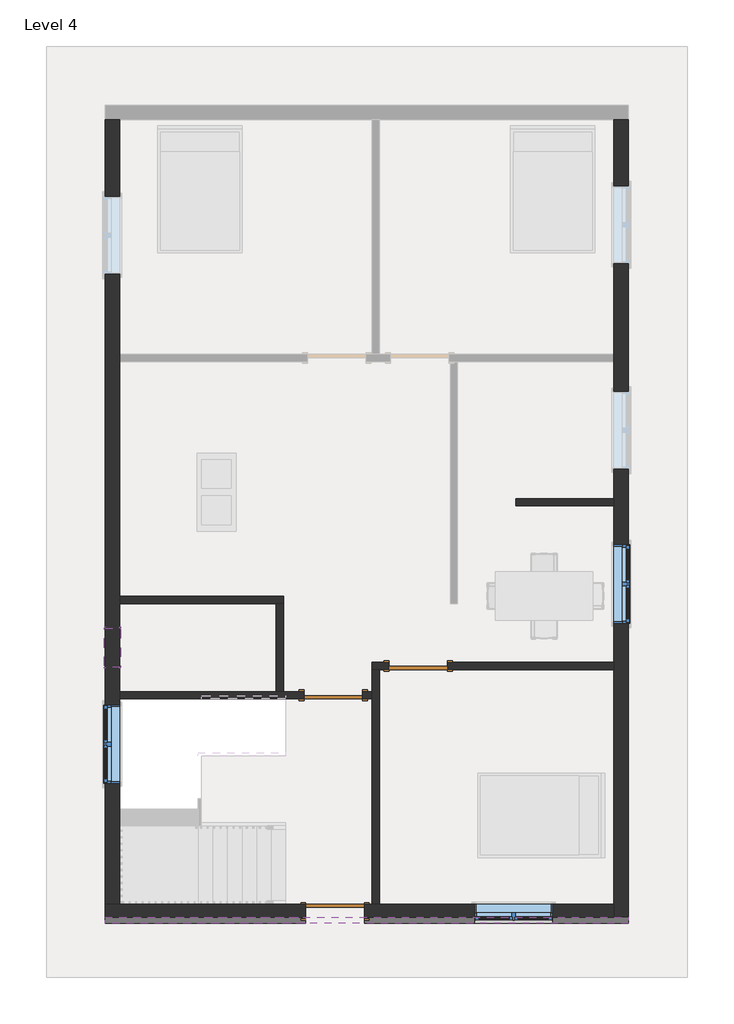
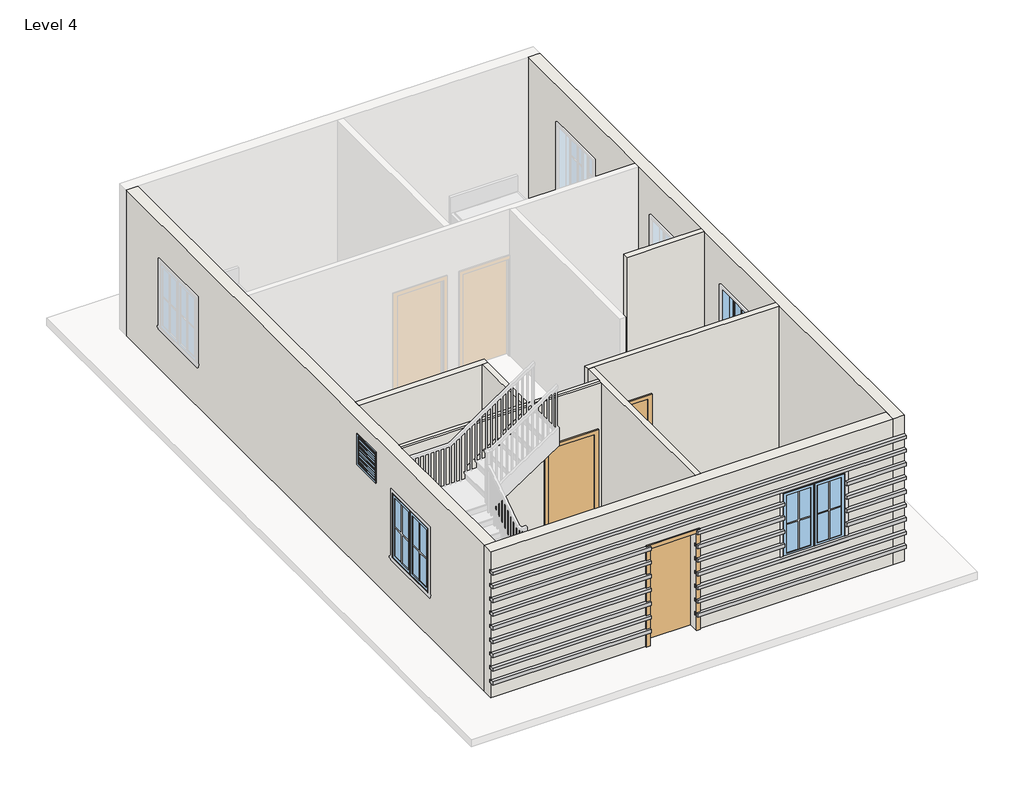
# One storey, part 1 of 3: 9 proxies, 9 walls, 4 windows, 3 doors.
"""IFC4 building model written with IfcOpenShell, lengths in millimetres."""

from ifc_helpers import new_model, si_unit, frame, origin, place, context, project, spatial, polyline, outline, extrude, faceted_brep, transform, mapped, element, save
from components import single_flush_door_3_17d80c48, single_flush_door_3_5e62189b, single_flush_door_3_89fc3733, window_casement_double_window_4_576b2d2c, window_f2d8fef0

model = new_model("IFC4")

# Units and contexts
model_context = context("Model", 3, world=origin())
ifc_project = project(units=[si_unit("LENGTHUNIT", "METRE", prefix="MILLI")], contexts=[model_context])

# Site, building, storey
site = spatial("IfcSite", under=ifc_project)
building = spatial("IfcBuilding", under=site)
storey = spatial("IfcBuildingStorey", under=building, Name="Level 4", Elevation=9448.8)

# Proxies
placement = place(None, origin())
element("IfcBuildingElementProxy", 1, Name="Reveal", ObjectType="Reveal", at=placement, inside=storey, context=model_context, shape_type="SweptSolid", body=[
    extrude(outline(polyline([(2831.4882597, -6585.4426559), (2831.4882597, -6677.5176559), (-1289.6617403, -6677.5176559), (-1289.6617403, -6585.4426559), (2831.4882597, -6585.4426559)])), frame((0.0, 0.0, 9753.6), z_axis=(0.0, 0.0, 1.0), x_axis=(1.0, 0.0, 0.0)), (0.0, 0.0, 1.0), 67.7333333),
    extrude(outline(polyline([(-2204.0617403, -6585.4426559), (-2204.0617403, -6677.5176559), (-5334.6117403, -6677.5176559), (-5334.6117403, -6585.4426559), (-2204.0617403, -6585.4426559)])), frame((0.0, 0.0, 9753.6), z_axis=(0.0, 0.0, 1.0), x_axis=(1.0, 0.0, 0.0)), (0.0, 0.0, 1.0), 67.7333333),
])
element("IfcBuildingElementProxy", 2, Name="Reveal", ObjectType="Reveal", at=placement, inside=storey, context=model_context, shape_type="SweptSolid", body=[
    extrude(outline(polyline([(2831.4882597, -6585.4426559), (2831.4882597, -6677.5176559), (-1289.6617403, -6677.5176559), (-1289.6617403, -6585.4426559), (2831.4882597, -6585.4426559)])), frame((0.0, 0.0, 10040.0994231), z_axis=(0.0, 0.0, 1.0), x_axis=(1.0, 0.0, 0.0)), (0.0, 0.0, 1.0), 67.7333333),
    extrude(outline(polyline([(-2204.0617403, -6585.4426559), (-2204.0617403, -6677.5176559), (-5334.6117403, -6677.5176559), (-5334.6117403, -6585.4426559), (-2204.0617403, -6585.4426559)])), frame((0.0, 0.0, 10040.0994231), z_axis=(0.0, 0.0, 1.0), x_axis=(1.0, 0.0, 0.0)), (0.0, 0.0, 1.0), 67.7333333),
])
element("IfcBuildingElementProxy", 3, Name="Reveal", ObjectType="Reveal", at=placement, inside=storey, context=model_context, shape_type="SweptSolid", body=[
    extrude(outline(polyline([(2831.4882597, -6585.4426559), (2831.4882597, -6677.5176559), (-1289.6617403, -6677.5176559), (-1289.6617403, -6585.4426559), (2831.4882597, -6585.4426559)])), frame((0.0, 0.0, 10326.5988461), z_axis=(0.0, 0.0, 1.0), x_axis=(1.0, 0.0, 0.0)), (0.0, 0.0, 1.0), 67.7333333),
    extrude(outline(polyline([(-2204.0617403, -6585.4426559), (-2204.0617403, -6677.5176559), (-5334.6117403, -6677.5176559), (-5334.6117403, -6585.4426559), (-2204.0617403, -6585.4426559)])), frame((0.0, 0.0, 10326.5988461), z_axis=(0.0, 0.0, 1.0), x_axis=(1.0, 0.0, 0.0)), (0.0, 0.0, 1.0), 67.7333333),
])
element("IfcBuildingElementProxy", 4, Name="Reveal", ObjectType="Reveal", at=placement, inside=storey, context=model_context, shape_type="SweptSolid", body=[
    extrude(outline(polyline([(2831.4882597, -6585.4426559), (2831.4882597, -6677.5176559), (1650.3882597, -6677.5176559), (1650.3882597, -6585.4426559), (2831.4882597, -6585.4426559)])), frame((0.0, 0.0, 10613.0982692), z_axis=(0.0, 0.0, 1.0), x_axis=(1.0, 0.0, 0.0)), (0.0, 0.0, 1.0), 67.7333333),
    extrude(outline(polyline([(431.1882597, -6585.4426559), (431.1882597, -6677.5176559), (-1289.6617403, -6677.5176559), (-1289.6617403, -6585.4426559), (431.1882597, -6585.4426559)])), frame((0.0, 0.0, 10613.0982692), z_axis=(0.0, 0.0, 1.0), x_axis=(1.0, 0.0, 0.0)), (0.0, 0.0, 1.0), 67.7333333),
    extrude(outline(polyline([(-2204.0617403, -6585.4426559), (-2204.0617403, -6677.5176559), (-5334.6117403, -6677.5176559), (-5334.6117403, -6585.4426559), (-2204.0617403, -6585.4426559)])), frame((0.0, 0.0, 10613.0982692), z_axis=(0.0, 0.0, 1.0), x_axis=(1.0, 0.0, 0.0)), (0.0, 0.0, 1.0), 67.7333333),
])
element("IfcBuildingElementProxy", 5, Name="Reveal", ObjectType="Reveal", at=placement, inside=storey, context=model_context, shape_type="SweptSolid", body=[
    extrude(outline(polyline([(2831.4882597, -6585.4426559), (2831.4882597, -6677.5176559), (1650.3882597, -6677.5176559), (1650.3882597, -6585.4426559), (2831.4882597, -6585.4426559)])), frame((0.0, 0.0, 10899.5976923), z_axis=(0.0, 0.0, 1.0), x_axis=(1.0, 0.0, 0.0)), (0.0, 0.0, 1.0), 67.7333333),
    extrude(outline(polyline([(431.1882597, -6585.4426559), (431.1882597, -6677.5176559), (-1289.6617403, -6677.5176559), (-1289.6617403, -6585.4426559), (431.1882597, -6585.4426559)])), frame((0.0, 0.0, 10899.5976923), z_axis=(0.0, 0.0, 1.0), x_axis=(1.0, 0.0, 0.0)), (0.0, 0.0, 1.0), 67.7333333),
    extrude(outline(polyline([(-2204.0617403, -6585.4426559), (-2204.0617403, -6677.5176559), (-5334.6117403, -6677.5176559), (-5334.6117403, -6585.4426559), (-2204.0617403, -6585.4426559)])), frame((0.0, 0.0, 10899.5976923), z_axis=(0.0, 0.0, 1.0), x_axis=(1.0, 0.0, 0.0)), (0.0, 0.0, 1.0), 67.7333333),
])
element("IfcBuildingElementProxy", 6, Name="Reveal", ObjectType="Reveal", at=placement, inside=storey, context=model_context, shape_type="SweptSolid", body=[
    extrude(outline(polyline([(2831.4882597, -6585.4426559), (2831.4882597, -6677.5176559), (1650.3882597, -6677.5176559), (1650.3882597, -6585.4426559), (2831.4882597, -6585.4426559)])), frame((0.0, 0.0, 11186.0971154), z_axis=(0.0, 0.0, 1.0), x_axis=(1.0, 0.0, 0.0)), (0.0, 0.0, 1.0), 67.7333333),
    extrude(outline(polyline([(431.1882597, -6585.4426559), (431.1882597, -6677.5176559), (-1289.6617403, -6677.5176559), (-1289.6617403, -6585.4426559), (431.1882597, -6585.4426559)])), frame((0.0, 0.0, 11186.0971154), z_axis=(0.0, 0.0, 1.0), x_axis=(1.0, 0.0, 0.0)), (0.0, 0.0, 1.0), 67.7333333),
    extrude(outline(polyline([(-2204.0617403, -6585.4426559), (-2204.0617403, -6677.5176559), (-5334.6117403, -6677.5176559), (-5334.6117403, -6585.4426559), (-2204.0617403, -6585.4426559)])), frame((0.0, 0.0, 11186.0971154), z_axis=(0.0, 0.0, 1.0), x_axis=(1.0, 0.0, 0.0)), (0.0, 0.0, 1.0), 67.7333333),
])
element("IfcBuildingElementProxy", 7, Name="Reveal", ObjectType="Reveal", at=placement, inside=storey, context=model_context, shape_type="SweptSolid", body=[
    extrude(outline(polyline([(2831.4882597, -6585.4426559), (2831.4882597, -6677.5176559), (1650.3882597, -6677.5176559), (1650.3882597, -6585.4426559), (2831.4882597, -6585.4426559)])), frame((0.0, 0.0, 11472.5965384), z_axis=(0.0, 0.0, 1.0), x_axis=(1.0, 0.0, 0.0)), (0.0, 0.0, 1.0), 67.7333333),
    extrude(outline(polyline([(431.1882597, -6585.4426559), (431.1882597, -6677.5176559), (-1289.6617403, -6677.5176559), (-1289.6617403, -6585.4426559), (431.1882597, -6585.4426559)])), frame((0.0, 0.0, 11472.5965384), z_axis=(0.0, 0.0, 1.0), x_axis=(1.0, 0.0, 0.0)), (0.0, 0.0, 1.0), 67.7333333),
    extrude(outline(polyline([(-2204.0617403, -6585.4426559), (-2204.0617403, -6677.5176559), (-5334.6117403, -6677.5176559), (-5334.6117403, -6585.4426559), (-2204.0617403, -6585.4426559)])), frame((0.0, 0.0, 11472.5965384), z_axis=(0.0, 0.0, 1.0), x_axis=(1.0, 0.0, 0.0)), (0.0, 0.0, 1.0), 67.7333333),
])
element("IfcBuildingElementProxy", 8, Name="Reveal", ObjectType="Reveal", at=placement, inside=storey, context=model_context, shape_type="SweptSolid", body=[
    extrude(outline(polyline([(2831.4882597, -6585.4426559), (2831.4882597, -6677.5176559), (-5334.6117403, -6677.5176559), (-5334.6117403, -6585.4426559), (2831.4882597, -6585.4426559)])), frame((0.0, 0.0, 11759.0959615), z_axis=(0.0, 0.0, 1.0), x_axis=(1.0, 0.0, 0.0)), (0.0, 0.0, 1.0), 67.7333333),
])
element("IfcBuildingElementProxy", 9, Name="Reveal", ObjectType="Reveal", at=placement, inside=storey, context=model_context, shape_type="SweptSolid", body=[
    extrude(outline(polyline([(2831.4882597, -6585.4426559), (2831.4882597, -6677.5176559), (-5334.6117403, -6677.5176559), (-5334.6117403, -6585.4426559), (2831.4882597, -6585.4426559)])), frame((0.0, 0.0, 12045.5953846), z_axis=(0.0, 0.0, 1.0), x_axis=(1.0, 0.0, 0.0)), (0.0, 0.0, 1.0), 67.7333333),
])

# Doors
single_flush_door_3_shape = single_flush_door_3_17d80c48(model_context)
element("IfcDoor", 10, ObjectType="Single-Flush : DOOR 3'", at=placement, inside=storey, context=model_context, shape_type="MappedRepresentation", body=[
    mapped(single_flush_door_3_shape, transform((-451.4617403, -2667.4926559, 9448.8), x_axis=(-1.0, 0.0, 0.0), y_axis=(0.0, -1.0, 0.0), z_axis=(0.0, 0.0, 1.0))),
])
single_flush_door_3_2_shape = single_flush_door_3_5e62189b(model_context)
element("IfcDoor", 11, ObjectType="Single-Flush : DOOR 3'", at=placement, inside=storey, context=model_context, shape_type="MappedRepresentation", body=[
    mapped(single_flush_door_3_2_shape, transform((-1772.2617403, -3124.6926559, 9448.8), x_axis=(1.0, 0.0, 0.0), y_axis=(0.0, 1.0, 0.0), z_axis=(0.0, 0.0, 1.0))),
])
single_flush_door_3_3_shape = single_flush_door_3_89fc3733(model_context)
element("IfcDoor", 12, ObjectType="Single-Flush : DOOR 3'", at=placement, inside=storey, context=model_context, shape_type="MappedRepresentation", body=[
    mapped(single_flush_door_3_3_shape, transform((-1746.8617403, -6496.5426559, 9448.8), x_axis=(1.0, 0.0, 0.0), y_axis=(0.0, 1.0, 0.0), z_axis=(0.0, 0.0, 1.0))),
])

# Walls
element("IfcWall", 13, ObjectType="ALL 4.5\"", at=placement, inside=storey, context=model_context, shape_type="SweptSolid", body=[
    extrude(outline(polyline([(1078.8882597, -57.6426559), (2602.8882597, -57.6426559), (2602.8882597, -171.9426559), (1078.8882597, -171.9426559), (1078.8882597, -57.6426559)])), frame((0.0, 0.0, 9448.8), z_axis=(0.0, 0.0, 1.0), x_axis=(1.0, 0.0, 0.0)), (0.0, 0.0, 1.0), 3048.0),
])
element("IfcWall", 14, ObjectType="ALL 4.5\"", at=placement, inside=storey, context=model_context, shape_type="Brep", body=[
    faceted_brep([(-908.6617403, -2610.3426559, 11480.8), (-908.6617403, -2610.3426559, 9448.8), (-1169.0117403, -2610.3426559, 9448.8), (-1169.0117403, -2610.3426559, 12496.8), (2602.8882597, -2610.3426559, 12496.8), (2602.8882597, -2610.3426559, 9448.8), (5.7382597, -2610.3426559, 9448.8), (5.7382597, -2610.3426559, 11480.8), (-1169.0117403, -2724.6426559, 9448.8), (-1054.7117403, -2724.6426559, 9448.8), (-908.6617403, -2724.6426559, 9448.8), (-908.6617403, -2724.6426559, 11480.8), (5.7382597, -2724.6426559, 11480.8), (5.7382597, -2724.6426559, 9448.8), (2602.8882597, -2724.6426559, 9448.8), (2602.8882597, -2724.6426559, 12496.8), (-1054.7117403, -2724.6426559, 12496.8), (-1169.0117403, -2724.6426559, 12496.8)], [[[0, 1, 2, 3, 4, 5, 6, 7]], [[8, 9, 10, 11, 12, 13, 14, 15, 16, 17]], [[6, 5, 14, 13]], [[2, 1, 10, 9, 8]], [[5, 4, 15, 14]], [[3, 2, 8, 17]], [[11, 10, 1, 0]], [[12, 11, 0, 7]], [[13, 12, 7, 6]], [[4, 3, 17, 16, 15]]]),
])
element("IfcWall", 15, ObjectType="ALL 4.5\"", at=placement, inside=storey, context=model_context, shape_type="Brep", body=[
    faceted_brep([(-1169.0117403, -2724.6426559, 9448.8), (-1169.0117403, -3067.5426559, 9448.8), (-1169.0117403, -3181.8426559, 9448.8), (-1169.0117403, -6382.2426559, 9448.8), (-1169.0117403, -6382.2426559, 12496.8), (-1169.0117403, -3181.8426559, 12496.8), (-1169.0117403, -3067.5426559, 12496.8), (-1169.0117403, -2724.6426559, 12496.8), (-1054.7117403, -2724.6426559, 9448.8), (-1054.7117403, -2724.6426559, 12496.8), (-1054.7117403, -6382.2426559, 12496.8), (-1054.7117403, -6382.2426559, 9448.8)], [[[0, 1, 2, 3, 4, 5, 6, 7]], [[8, 9, 10, 11]], [[3, 2, 1, 0, 8, 11]], [[0, 7, 9, 8]], [[4, 3, 11, 10]], [[7, 6, 5, 4, 10, 9]]]),
])
element("IfcWall", 16, ObjectType="ALL 4.5\"", at=placement, inside=storey, context=model_context, shape_type="Brep", body=[
    faceted_brep([(-1169.0117403, -3067.5426559, 9448.8), (-1315.0617403, -3067.5426559, 9448.8), (-1315.0617403, -3067.5426559, 11480.8), (-2229.4617403, -3067.5426559, 11480.8), (-2229.4617403, -3067.5426559, 9448.8), (-2553.3117403, -3067.5426559, 9448.8), (-2667.6117403, -3067.5426559, 9448.8), (-5106.0117403, -3067.5426559, 9448.8), (-5106.0117403, -3067.5426559, 12496.8), (-2667.6117403, -3067.5426559, 12496.8), (-2553.3117403, -3067.5426559, 12496.8), (-1169.0117403, -3067.5426559, 12496.8), (-1315.0617403, -3181.8426559, 11480.8), (-1315.0617403, -3181.8426559, 9448.8), (-1169.0117403, -3181.8426559, 9448.8), (-1169.0117403, -3181.8426559, 12496.8), (-5106.0117403, -3181.8426559, 12496.8), (-5106.0117403, -3181.8426559, 9448.8), (-2229.4617403, -3181.8426559, 9448.8), (-2229.4617403, -3181.8426559, 11480.8), (-5106.0117403, -3131.0426559, 12496.8), (-1169.0117403, -3131.0426559, 12496.8), (-2515.2117403, -3131.0426559, 12496.8)], [[[0, 1, 2, 3, 4, 5, 6, 7, 8, 9, 10, 11]], [[12, 13, 14, 15, 16, 17, 18, 19]], [[18, 17, 7, 6, 5, 4]], [[14, 13, 1, 0]], [[8, 7, 17, 16, 20]], [[0, 11, 21, 15, 14]], [[2, 1, 13, 12]], [[3, 2, 12, 19]], [[4, 3, 19, 18]], [[11, 10, 9, 8, 20, 22, 21]], [[20, 16, 15, 21, 22]]]),
])
element("IfcWall", 17, ObjectType="ALL 4.5\"", at=placement, inside=storey, context=model_context, shape_type="Brep", body=[
    faceted_brep([(-5106.0117403, -1695.9426559, 9448.8), (-2667.6117403, -1695.9426559, 9448.8), (-2553.3117403, -1695.9426559, 9448.8), (-2553.3117403, -1695.9426559, 12496.8), (-2667.6117403, -1695.9426559, 12496.8), (-5106.0117403, -1695.9426559, 12496.8), (-5106.0117403, -1581.6426559, 9448.8), (-5106.0117403, -1581.6426559, 12496.8), (-2553.3117403, -1581.6426559, 12496.8), (-2553.3117403, -1581.6426559, 9448.8)], [[[0, 1, 2, 3, 4, 5]], [[6, 7, 8, 9]], [[2, 1, 0, 6, 9]], [[0, 5, 7, 6]], [[3, 2, 9, 8]], [[5, 4, 3, 8, 7]]]),
])
element("IfcWall", 18, ObjectType="ALL 4.5\"", at=placement, inside=storey, context=model_context, shape_type="SweptSolid", body=[
    extrude(outline(polyline([(-2667.6117403, -3067.5426559), (-2667.6117403, -1695.9426559), (-2553.3117403, -1695.9426559), (-2553.3117403, -3067.5426559), (-2667.6117403, -3067.5426559)])), frame((0.0, 0.0, 9448.8), z_axis=(0.0, 0.0, 1.0), x_axis=(1.0, 0.0, 0.0)), (0.0, 0.0, 1.0), 3048.0),
])
element("IfcWall", 19, ObjectType="WALL 9\"", at=placement, inside=storey, context=model_context, shape_type="Brep", body=[
    faceted_brep([(2602.8882597, 5847.8573441, 9448.8), (2602.8882597, 2190.2573441, 9448.8), (2602.8882597, 2075.9573441, 9448.8), (2602.8882597, -57.6426559, 9448.8), (2602.8882597, -171.9426559, 9448.8), (2602.8882597, -2610.3426559, 9448.8), (2602.8882597, -2724.6426559, 9448.8), (2602.8882597, -6382.2426559, 9448.8), (2602.8882597, -6610.8426559, 9448.8), (2602.8882597, -6610.8426559, 9753.6), (2602.8882597, -6585.4426559, 9753.6), (2602.8882597, -6585.4426559, 9821.3333333), (2602.8882597, -6610.8426559, 9821.3333333), (2602.8882597, -6610.8426559, 10040.0994231), (2602.8882597, -6585.4426559, 10040.0994231), (2602.8882597, -6585.4426559, 10107.8327564), (2602.8882597, -6610.8426559, 10107.8327564), (2602.8882597, -6610.8426559, 10326.5988461), (2602.8882597, -6585.4426559, 10326.5988461), (2602.8882597, -6585.4426559, 10394.3321795), (2602.8882597, -6610.8426559, 10394.3321795), (2602.8882597, -6610.8426559, 10613.0982692), (2602.8882597, -6585.4426559, 10613.0982692), (2602.8882597, -6585.4426559, 10680.8316025), (2602.8882597, -6610.8426559, 10680.8316025), (2602.8882597, -6610.8426559, 10899.5976923), (2602.8882597, -6585.4426559, 10899.5976923), (2602.8882597, -6585.4426559, 10967.3310256), (2602.8882597, -6610.8426559, 10967.3310256), (2602.8882597, -6610.8426559, 11186.0971154), (2602.8882597, -6585.4426559, 11186.0971154), (2602.8882597, -6585.4426559, 11253.8304487), (2602.8882597, -6610.8426559, 11253.8304487), (2602.8882597, -6610.8426559, 11472.5965384), (2602.8882597, -6585.4426559, 11472.5965384), (2602.8882597, -6585.4426559, 11540.3298718), (2602.8882597, -6610.8426559, 11540.3298718), (2602.8882597, -6610.8426559, 11759.0959615), (2602.8882597, -6585.4426559, 11759.0959615), (2602.8882597, -6585.4426559, 11826.8292948), (2602.8882597, -6610.8426559, 11826.8292948), (2602.8882597, -6610.8426559, 12045.5953846), (2602.8882597, -6585.4426559, 12045.5953846), (2602.8882597, -6585.4426559, 12113.3287179), (2602.8882597, -6610.8426559, 12113.3287179), (2602.8882597, -6610.8426559, 12496.8), (2602.8882597, -6382.2426559, 12496.8), (2602.8882597, -2724.6426559, 12496.8), (2602.8882597, -2610.3426559, 12496.8), (2602.8882597, -171.9426559, 12496.8), (2602.8882597, -57.6426559, 12496.8), (2602.8882597, 2075.9573441, 12496.8), (2602.8882597, 2190.2573441, 12496.8), (2602.8882597, 5847.8573441, 12496.8), (2602.8882597, 3599.9573441, 11709.4), (2602.8882597, 3599.9573441, 10363.2), (2602.8882597, 4819.1573441, 10363.2), (2602.8882597, 4819.1573441, 11709.4), (2602.8882597, 399.5573441, 11709.4), (2602.8882597, 399.5573441, 10363.2), (2602.8882597, 1618.7573441, 10363.2), (2602.8882597, 1618.7573441, 11709.4), (2602.8882597, -2000.7426559, 11709.4), (2602.8882597, -2000.7426559, 10363.2), (2602.8882597, -781.5426559, 10363.2), (2602.8882597, -781.5426559, 11709.4), (2831.4882597, -6610.8426559, 9448.8), (2831.4882597, 5847.8573441, 9448.8), (2831.4882597, 5847.8573441, 12496.8), (2831.4882597, -6610.8426559, 12496.8), (2831.4882597, -6610.8426559, 12113.3287179), (2831.4882597, -6585.4426559, 12113.3287179), (2831.4882597, -6585.4426559, 12045.5953846), (2831.4882597, -6610.8426559, 12045.5953846), (2831.4882597, -6610.8426559, 11826.8292948), (2831.4882597, -6585.4426559, 11826.8292948), (2831.4882597, -6585.4426559, 11759.0959615), (2831.4882597, -6610.8426559, 11759.0959615), (2831.4882597, -6610.8426559, 11540.3298718), (2831.4882597, -6585.4426559, 11540.3298718), (2831.4882597, -6585.4426559, 11472.5965384), (2831.4882597, -6610.8426559, 11472.5965384), (2831.4882597, -6610.8426559, 11253.8304487), (2831.4882597, -6585.4426559, 11253.8304487), (2831.4882597, -6585.4426559, 11186.0971154), (2831.4882597, -6610.8426559, 11186.0971154), (2831.4882597, -6610.8426559, 10967.3310256), (2831.4882597, -6585.4426559, 10967.3310256), (2831.4882597, -6585.4426559, 10899.5976923), (2831.4882597, -6610.8426559, 10899.5976923), (2831.4882597, -6610.8426559, 10680.8316025), (2831.4882597, -6585.4426559, 10680.8316025), (2831.4882597, -6585.4426559, 10613.0982692), (2831.4882597, -6610.8426559, 10613.0982692), (2831.4882597, -6610.8426559, 10394.3321795), (2831.4882597, -6585.4426559, 10394.3321795), (2831.4882597, -6585.4426559, 10326.5988461), (2831.4882597, -6610.8426559, 10326.5988461), (2831.4882597, -6610.8426559, 10107.8327564), (2831.4882597, -6585.4426559, 10107.8327564), (2831.4882597, -6585.4426559, 10040.0994231), (2831.4882597, -6610.8426559, 10040.0994231), (2831.4882597, -6610.8426559, 9821.3333333), (2831.4882597, -6585.4426559, 9821.3333333), (2831.4882597, -6585.4426559, 9753.6), (2831.4882597, -6610.8426559, 9753.6), (2831.4882597, 3599.9573441, 10363.2), (2831.4882597, 3599.9573441, 11709.4), (2831.4882597, 4819.1573441, 11709.4), (2831.4882597, 4819.1573441, 10363.2), (2831.4882597, 399.5573441, 10363.2), (2831.4882597, 399.5573441, 11709.4), (2831.4882597, 1618.7573441, 11709.4), (2831.4882597, 1618.7573441, 10363.2), (2831.4882597, -2000.7426559, 10363.2), (2831.4882597, -2000.7426559, 11709.4), (2831.4882597, -781.5426559, 11709.4), (2831.4882597, -781.5426559, 10363.2)], [[[0, 1, 2, 3, 4, 5, 6, 7, 8, 9, 10, 11, 12, 13, 14, 15, 16, 17, 18, 19, 20, 21, 22, 23, 24, 25, 26, 27, 28, 29, 30, 31, 32, 33, 34, 35, 36, 37, 38, 39, 40, 41, 42, 43, 44, 45, 46, 47, 48, 49, 50, 51, 52, 53], [54, 55, 56, 57], [58, 59, 60, 61], [62, 63, 64, 65]], [[66, 67, 68, 69, 70, 71, 72, 73, 74, 75, 76, 77, 78, 79, 80, 81, 82, 83, 84, 85, 86, 87, 88, 89, 90, 91, 92, 93, 94, 95, 96, 97, 98, 99, 100, 101, 102, 103, 104, 105], [106, 107, 108, 109], [110, 111, 112, 113], [114, 115, 116, 117]], [[8, 7, 6, 5, 4, 3, 2, 1, 0, 67, 66]], [[0, 53, 68, 67]], [[8, 66, 105, 9]], [[69, 45, 44, 70]], [[12, 102, 101, 13]], [[16, 98, 97, 17]], [[20, 94, 93, 21]], [[24, 90, 89, 25]], [[28, 86, 85, 29]], [[32, 82, 81, 33]], [[36, 78, 77, 37]], [[40, 74, 73, 41]], [[55, 54, 107, 106]], [[56, 55, 106, 109]], [[57, 56, 109, 108]], [[54, 57, 108, 107]], [[59, 58, 111, 110]], [[60, 59, 110, 113]], [[61, 60, 113, 112]], [[58, 61, 112, 111]], [[63, 62, 115, 114]], [[64, 63, 114, 117]], [[65, 64, 117, 116]], [[62, 65, 116, 115]], [[53, 52, 51, 50, 49, 48, 47, 46, 45, 69, 68]], [[11, 103, 102, 12]], [[104, 10, 9, 105]], [[103, 11, 10, 104]], [[15, 99, 98, 16]], [[100, 14, 13, 101]], [[99, 15, 14, 100]], [[19, 95, 94, 20]], [[96, 18, 17, 97]], [[95, 19, 18, 96]], [[23, 91, 90, 24]], [[92, 22, 21, 93]], [[91, 23, 22, 92]], [[27, 87, 86, 28]], [[88, 26, 25, 89]], [[87, 27, 26, 88]], [[31, 83, 82, 32]], [[84, 30, 29, 85]], [[83, 31, 30, 84]], [[35, 79, 78, 36]], [[80, 34, 33, 81]], [[79, 35, 34, 80]], [[39, 75, 74, 40]], [[76, 38, 37, 77]], [[75, 39, 38, 76]], [[43, 71, 70, 44]], [[72, 42, 41, 73]], [[71, 43, 42, 72]]]),
])
element("IfcWall", 20, ObjectType="WALL 9\"", at=placement, inside=storey, context=model_context, shape_type="Brep", body=[
    faceted_brep([(-5334.6117403, -6382.2426559, 12496.8), (-5106.0117403, -6382.2426559, 12496.8), (-1169.0117403, -6382.2426559, 12496.8), (-1054.7117403, -6382.2426559, 12496.8), (2602.8882597, -6382.2426559, 12496.8), (2602.8882597, -6382.2426559, 9448.8), (-1054.7117403, -6382.2426559, 9448.8), (-1169.0117403, -6382.2426559, 9448.8), (-1289.6617403, -6382.2426559, 9448.8), (-1289.6617403, -6382.2426559, 11480.8), (-2204.0617403, -6382.2426559, 11480.8), (-2204.0617403, -6382.2426559, 9448.8), (-5106.0117403, -6382.2426559, 9448.8), (-5334.6117403, -6382.2426559, 9448.8), (431.1882597, -6382.2426559, 11709.4), (431.1882597, -6382.2426559, 10363.2), (1650.3882597, -6382.2426559, 10363.2), (1650.3882597, -6382.2426559, 11709.4), (2602.8882597, -6610.8426559, 12496.8), (-5334.6117403, -6610.8426559, 12496.8), (-5334.6117403, -6610.8426559, 12113.3287179), (2602.8882597, -6610.8426559, 12113.3287179), (431.1882597, -6610.8426559, 11709.4), (1650.3882597, -6610.8426559, 11709.4), (1650.3882597, -6610.8426559, 11540.3298718), (2602.8882597, -6610.8426559, 11540.3298718), (2602.8882597, -6610.8426559, 11759.0959615), (-5334.6117403, -6610.8426559, 11759.0959615), (-5334.6117403, -6610.8426559, 11540.3298718), (-2204.0617403, -6610.8426559, 11540.3298718), (-2204.0617403, -6610.8426559, 11480.8), (-1289.6617403, -6610.8426559, 11480.8), (-1289.6617403, -6610.8426559, 11540.3298718), (431.1882597, -6610.8426559, 11540.3298718), (-5334.6117403, -6610.8426559, 9448.8), (-2204.0617403, -6610.8426559, 9448.8), (-2204.0617403, -6610.8426559, 9753.6), (-5334.6117403, -6610.8426559, 9753.6), (-1289.6617403, -6610.8426559, 9448.8), (2602.8882597, -6610.8426559, 9448.8), (2602.8882597, -6610.8426559, 9753.6), (-1289.6617403, -6610.8426559, 9753.6), (-1289.6617403, -6610.8426559, 9821.3333333), (2602.8882597, -6610.8426559, 9821.3333333), (2602.8882597, -6610.8426559, 10040.0994231), (-1289.6617403, -6610.8426559, 10040.0994231), (-5334.6117403, -6610.8426559, 9821.3333333), (-2204.0617403, -6610.8426559, 9821.3333333), (-2204.0617403, -6610.8426559, 10040.0994231), (-5334.6117403, -6610.8426559, 10040.0994231), (-1289.6617403, -6610.8426559, 10107.8327564), (2602.8882597, -6610.8426559, 10107.8327564), (2602.8882597, -6610.8426559, 10326.5988461), (-1289.6617403, -6610.8426559, 10326.5988461), (-5334.6117403, -6610.8426559, 10107.8327564), (-2204.0617403, -6610.8426559, 10107.8327564), (-2204.0617403, -6610.8426559, 10326.5988461), (-5334.6117403, -6610.8426559, 10326.5988461), (-1289.6617403, -6610.8426559, 10394.3321795), (431.1882597, -6610.8426559, 10394.3321795), (431.1882597, -6610.8426559, 10613.0982692), (-1289.6617403, -6610.8426559, 10613.0982692), (1650.3882597, -6610.8426559, 10394.3321795), (2602.8882597, -6610.8426559, 10394.3321795), (2602.8882597, -6610.8426559, 10613.0982692), (1650.3882597, -6610.8426559, 10613.0982692), (-5334.6117403, -6610.8426559, 10394.3321795), (-2204.0617403, -6610.8426559, 10394.3321795), (-2204.0617403, -6610.8426559, 10613.0982692), (-5334.6117403, -6610.8426559, 10613.0982692), (1650.3882597, -6610.8426559, 10680.8316025), (2602.8882597, -6610.8426559, 10680.8316025), (2602.8882597, -6610.8426559, 10899.5976923), (1650.3882597, -6610.8426559, 10899.5976923), (-1289.6617403, -6610.8426559, 10680.8316025), (431.1882597, -6610.8426559, 10680.8316025), (431.1882597, -6610.8426559, 10899.5976923), (-1289.6617403, -6610.8426559, 10899.5976923), (-5334.6117403, -6610.8426559, 10680.8316025), (-2204.0617403, -6610.8426559, 10680.8316025), (-2204.0617403, -6610.8426559, 10899.5976923), (-5334.6117403, -6610.8426559, 10899.5976923), (1650.3882597, -6610.8426559, 10967.3310256), (2602.8882597, -6610.8426559, 10967.3310256), (2602.8882597, -6610.8426559, 11186.0971154), (1650.3882597, -6610.8426559, 11186.0971154), (-1289.6617403, -6610.8426559, 10967.3310256), (431.1882597, -6610.8426559, 10967.3310256), (431.1882597, -6610.8426559, 11186.0971154), (-1289.6617403, -6610.8426559, 11186.0971154), (-5334.6117403, -6610.8426559, 10967.3310256), (-2204.0617403, -6610.8426559, 10967.3310256), (-2204.0617403, -6610.8426559, 11186.0971154), (-5334.6117403, -6610.8426559, 11186.0971154), (1650.3882597, -6610.8426559, 11253.8304487), (2602.8882597, -6610.8426559, 11253.8304487), (2602.8882597, -6610.8426559, 11472.5965384), (1650.3882597, -6610.8426559, 11472.5965384), (-1289.6617403, -6610.8426559, 11253.8304487), (431.1882597, -6610.8426559, 11253.8304487), (431.1882597, -6610.8426559, 11472.5965384), (-1289.6617403, -6610.8426559, 11472.5965384), (-5334.6117403, -6610.8426559, 11253.8304487), (-2204.0617403, -6610.8426559, 11253.8304487), (-2204.0617403, -6610.8426559, 11472.5965384), (-5334.6117403, -6610.8426559, 11472.5965384), (-5334.6117403, -6610.8426559, 11826.8292948), (2602.8882597, -6610.8426559, 11826.8292948), (2602.8882597, -6610.8426559, 12045.5953846), (-5334.6117403, -6610.8426559, 12045.5953846), (2602.8882597, -6585.4426559, 12113.3287179), (2602.8882597, -6585.4426559, 12045.5953846), (2602.8882597, -6585.4426559, 11826.8292948), (2602.8882597, -6585.4426559, 11759.0959615), (2602.8882597, -6585.4426559, 11540.3298718), (2602.8882597, -6585.4426559, 11472.5965384), (2602.8882597, -6585.4426559, 11253.8304487), (2602.8882597, -6585.4426559, 11186.0971154), (2602.8882597, -6585.4426559, 10967.3310256), (2602.8882597, -6585.4426559, 10899.5976923), (2602.8882597, -6585.4426559, 10680.8316025), (2602.8882597, -6585.4426559, 10613.0982692), (2602.8882597, -6585.4426559, 10394.3321795), (2602.8882597, -6585.4426559, 10326.5988461), (2602.8882597, -6585.4426559, 10107.8327564), (2602.8882597, -6585.4426559, 10040.0994231), (2602.8882597, -6585.4426559, 9821.3333333), (2602.8882597, -6585.4426559, 9753.6), (-5334.6117403, -6585.4426559, 9753.6), (-5334.6117403, -6585.4426559, 9821.3333333), (-5334.6117403, -6585.4426559, 10040.0994231), (-5334.6117403, -6585.4426559, 10107.8327564), (-5334.6117403, -6585.4426559, 10326.5988461), (-5334.6117403, -6585.4426559, 10394.3321795), (-5334.6117403, -6585.4426559, 10613.0982692), (-5334.6117403, -6585.4426559, 10680.8316025), (-5334.6117403, -6585.4426559, 10899.5976923), (-5334.6117403, -6585.4426559, 10967.3310256), (-5334.6117403, -6585.4426559, 11186.0971154), (-5334.6117403, -6585.4426559, 11253.8304487), (-5334.6117403, -6585.4426559, 11472.5965384), (-5334.6117403, -6585.4426559, 11540.3298718), (-5334.6117403, -6585.4426559, 11759.0959615), (-5334.6117403, -6585.4426559, 11826.8292948), (-5334.6117403, -6585.4426559, 12045.5953846), (-5334.6117403, -6585.4426559, 12113.3287179), (431.1882597, -6585.4426559, 11540.3298718), (431.1882597, -6585.4426559, 11472.5965384), (431.1882597, -6585.4426559, 11253.8304487), (431.1882597, -6585.4426559, 11186.0971154), (431.1882597, -6585.4426559, 10967.3310256), (431.1882597, -6585.4426559, 10899.5976923), (431.1882597, -6585.4426559, 10680.8316025), (431.1882597, -6585.4426559, 10613.0982692), (431.1882597, -6585.4426559, 10394.3321795), (431.1882597, -6585.4426559, 10363.2), (1650.3882597, -6585.4426559, 10363.2), (1650.3882597, -6585.4426559, 10394.3321795), (1650.3882597, -6585.4426559, 10613.0982692), (1650.3882597, -6585.4426559, 10680.8316025), (1650.3882597, -6585.4426559, 10899.5976923), (1650.3882597, -6585.4426559, 10967.3310256), (1650.3882597, -6585.4426559, 11186.0971154), (1650.3882597, -6585.4426559, 11253.8304487), (1650.3882597, -6585.4426559, 11472.5965384), (1650.3882597, -6585.4426559, 11540.3298718), (-1289.6617403, -6585.4426559, 9753.6), (-1289.6617403, -6585.4426559, 9821.3333333), (-1289.6617403, -6585.4426559, 10040.0994231), (-1289.6617403, -6585.4426559, 10107.8327564), (-1289.6617403, -6585.4426559, 10326.5988461), (-1289.6617403, -6585.4426559, 10394.3321795), (-1289.6617403, -6585.4426559, 10613.0982692), (-1289.6617403, -6585.4426559, 10680.8316025), (-1289.6617403, -6585.4426559, 10899.5976923), (-1289.6617403, -6585.4426559, 10967.3310256), (-1289.6617403, -6585.4426559, 11186.0971154), (-1289.6617403, -6585.4426559, 11253.8304487), (-1289.6617403, -6585.4426559, 11472.5965384), (-1289.6617403, -6585.4426559, 11480.8), (-2204.0617403, -6585.4426559, 11480.8), (-2204.0617403, -6585.4426559, 11472.5965384), (-2204.0617403, -6585.4426559, 11253.8304487), (-2204.0617403, -6585.4426559, 11186.0971154), (-2204.0617403, -6585.4426559, 10967.3310256), (-2204.0617403, -6585.4426559, 10899.5976923), (-2204.0617403, -6585.4426559, 10680.8316025), (-2204.0617403, -6585.4426559, 10613.0982692), (-2204.0617403, -6585.4426559, 10394.3321795), (-2204.0617403, -6585.4426559, 10326.5988461), (-2204.0617403, -6585.4426559, 10107.8327564), (-2204.0617403, -6585.4426559, 10040.0994231), (-2204.0617403, -6585.4426559, 9821.3333333), (-2204.0617403, -6585.4426559, 9753.6), (-1289.6617403, -6585.4426559, 11540.3298718), (-2204.0617403, -6585.4426559, 11540.3298718)], [[[0, 1, 2, 3, 4, 5, 6, 7, 8, 9, 10, 11, 12, 13], [14, 15, 16, 17]], [[18, 19, 20, 21]], [[22, 23, 24, 25, 26, 27, 28, 29, 30, 31, 32, 33]], [[34, 35, 36, 37]], [[38, 39, 40, 41]], [[42, 43, 44, 45]], [[46, 47, 48, 49]], [[50, 51, 52, 53]], [[54, 55, 56, 57]], [[58, 59, 60, 61]], [[62, 63, 64, 65]], [[66, 67, 68, 69]], [[70, 71, 72, 73]], [[74, 75, 76, 77]], [[78, 79, 80, 81]], [[82, 83, 84, 85]], [[86, 87, 88, 89]], [[90, 91, 92, 93]], [[94, 95, 96, 97]], [[98, 99, 100, 101]], [[102, 103, 104, 105]], [[106, 107, 108, 109]], [[5, 39, 38, 8, 7, 6]], [[34, 13, 12, 11, 35]], [[4, 3, 2, 1, 0, 19, 18]], [[5, 4, 18, 21, 110, 111, 108, 107, 112, 113, 26, 25, 114, 115, 96, 95, 116, 117, 84, 83, 118, 119, 72, 71, 120, 121, 64, 63, 122, 123, 52, 51, 124, 125, 44, 43, 126, 127, 40, 39]], [[0, 13, 34, 37, 128, 129, 46, 49, 130, 131, 54, 57, 132, 133, 66, 69, 134, 135, 78, 81, 136, 137, 90, 93, 138, 139, 102, 105, 140, 141, 28, 27, 142, 143, 106, 109, 144, 145, 20, 19]], [[15, 14, 22, 33, 146, 147, 100, 99, 148, 149, 88, 87, 150, 151, 76, 75, 152, 153, 60, 59, 154, 155]], [[16, 15, 155, 156]], [[17, 16, 156, 157, 62, 65, 158, 159, 70, 73, 160, 161, 82, 85, 162, 163, 94, 97, 164, 165, 24, 23]], [[14, 17, 23, 22]], [[9, 8, 38, 41, 166, 167, 42, 45, 168, 169, 50, 53, 170, 171, 58, 61, 172, 173, 74, 77, 174, 175, 86, 89, 176, 177, 98, 101, 178, 179]], [[10, 9, 179, 31, 30, 180]], [[11, 10, 180, 181, 104, 103, 182, 183, 92, 91, 184, 185, 80, 79, 186, 187, 68, 67, 188, 189, 56, 55, 190, 191, 48, 47, 192, 193, 36, 35]], [[167, 126, 43, 42]], [[127, 166, 41, 40]], [[126, 167, 166, 127]], [[129, 192, 47, 46]], [[193, 128, 37, 36]], [[192, 129, 128, 193]], [[169, 124, 51, 50]], [[125, 168, 45, 44]], [[124, 169, 168, 125]], [[131, 190, 55, 54]], [[191, 130, 49, 48]], [[190, 131, 130, 191]], [[171, 154, 59, 58]], [[157, 122, 63, 62]], [[123, 170, 53, 52]], [[154, 171, 170, 123, 122, 157, 156, 155]], [[133, 188, 67, 66]], [[189, 132, 57, 56]], [[188, 133, 132, 189]], [[159, 120, 71, 70]], [[121, 158, 65, 64]], [[120, 159, 158, 121]], [[173, 152, 75, 74]], [[153, 172, 61, 60]], [[152, 173, 172, 153]], [[135, 186, 79, 78]], [[187, 134, 69, 68]], [[186, 135, 134, 187]], [[161, 118, 83, 82]], [[119, 160, 73, 72]], [[118, 161, 160, 119]], [[175, 150, 87, 86]], [[151, 174, 77, 76]], [[150, 175, 174, 151]], [[137, 184, 91, 90]], [[185, 136, 81, 80]], [[184, 137, 136, 185]], [[163, 116, 95, 94]], [[117, 162, 85, 84]], [[116, 163, 162, 117]], [[177, 148, 99, 98]], [[149, 176, 89, 88]], [[148, 177, 176, 149]], [[139, 182, 103, 102]], [[183, 138, 93, 92]], [[182, 139, 138, 183]], [[165, 114, 25, 24]], [[115, 164, 97, 96]], [[114, 165, 164, 115]], [[179, 194, 32, 31]], [[194, 146, 33, 32]], [[147, 178, 101, 100]], [[146, 194, 179, 178, 147]], [[195, 180, 30, 29]], [[141, 195, 29, 28]], [[181, 140, 105, 104]], [[195, 141, 140, 181, 180]], [[143, 112, 107, 106]], [[113, 142, 27, 26]], [[112, 143, 142, 113]], [[145, 110, 21, 20]], [[111, 144, 109, 108]], [[110, 145, 144, 111]]]),
])
element("IfcWall", 21, ObjectType="WALL 9\"", at=placement, inside=storey, context=model_context, shape_type="Brep", body=[
    faceted_brep([(-5106.0117403, -6382.2426559, 9448.8), (-5106.0117403, -3181.8426559, 9448.8), (-5106.0117403, -3067.5426559, 9448.8), (-5106.0117403, -1695.9426559, 9448.8), (-5106.0117403, -1581.6426559, 9448.8), (-5106.0117403, 2075.9573441, 9448.8), (-5106.0117403, 2190.2573441, 9448.8), (-5106.0117403, 5847.8573441, 9448.8), (-5106.0117403, 5847.8573441, 12496.8), (-5106.0117403, 2190.2573441, 12496.8), (-5106.0117403, 2075.9573441, 12496.8), (-5106.0117403, -1581.6426559, 12496.8), (-5106.0117403, -1695.9426559, 12496.8), (-5106.0117403, -3067.5426559, 12496.8), (-5106.0117403, -3181.8426559, 12496.8), (-5106.0117403, -6382.2426559, 12496.8), (-5106.0117403, -3277.0926559, 11709.4), (-5106.0117403, -3277.0926559, 10363.2), (-5106.0117403, -4496.2926559, 10363.2), (-5106.0117403, -4496.2926559, 11709.4), (-5106.0117403, 4657.2323441, 11709.4), (-5106.0117403, 4657.2323441, 10363.2), (-5106.0117403, 3438.0323441, 10363.2), (-5106.0117403, 3438.0323441, 11709.4), (-5106.0117403, -2686.5426559, 12192.0), (-5106.0117403, -2076.9426559, 12192.0), (-5106.0117403, -2076.9426559, 11582.4), (-5106.0117403, -2686.5426559, 11582.4), (-5334.6117403, -6382.2426559, 9448.8), (-5334.6117403, -6382.2426559, 12496.8), (-5334.6117403, 5847.8573441, 12496.8), (-5334.6117403, 5847.8573441, 9448.8), (-5334.6117403, -3277.0926559, 11709.4), (-5334.6117403, -4496.2926559, 11709.4), (-5334.6117403, -4496.2926559, 10363.2), (-5334.6117403, -3277.0926559, 10363.2), (-5334.6117403, 4657.2323441, 11709.4), (-5334.6117403, 3438.0323441, 11709.4), (-5334.6117403, 3438.0323441, 10363.2), (-5334.6117403, 4657.2323441, 10363.2), (-5334.6117403, -2686.5426559, 12192.0), (-5334.6117403, -2686.5426559, 11582.4), (-5334.6117403, -2076.9426559, 11582.4), (-5334.6117403, -2076.9426559, 12192.0)], [[[0, 1, 2, 3, 4, 5, 6, 7, 8, 9, 10, 11, 12, 13, 14, 15], [16, 17, 18, 19], [20, 21, 22, 23], [24, 25, 26, 27]], [[28, 29, 30, 31], [32, 33, 34, 35], [36, 37, 38, 39], [40, 41, 42, 43]], [[7, 6, 5, 4, 3, 2, 1, 0, 28, 31]], [[15, 14, 13, 12, 11, 10, 9, 8, 30, 29]], [[8, 7, 31, 30]], [[0, 15, 29, 28]], [[17, 16, 32, 35]], [[18, 17, 35, 34]], [[19, 18, 34, 33]], [[16, 19, 33, 32]], [[21, 20, 36, 39]], [[22, 21, 39, 38]], [[23, 22, 38, 37]], [[20, 23, 37, 36]], [[41, 40, 24, 27]], [[42, 41, 27, 26]], [[43, 42, 26, 25]], [[40, 43, 25, 24]]]),
])

# Windows
window_casement_double_window_4_shape = window_casement_double_window_4_576b2d2c(model_context)
element("IfcWindow", 22, ObjectType="Window-Casement-Double : WINDOW 4'", at=placement, inside=storey, context=model_context, shape_type="MappedRepresentation", body=[
    mapped(window_casement_double_window_4_shape, transform((-5220.3117403, -3886.6926559, 9448.8), x_axis=(0.0, 1.0, 0.0), y_axis=(-1.0, 0.0, 0.0), z_axis=(0.0, 0.0, 1.0))),
])
element("IfcWindow", 23, ObjectType="Window-Casement-Double : WINDOW 4'", at=placement, inside=storey, context=model_context, shape_type="MappedRepresentation", body=[
    mapped(window_casement_double_window_4_shape, transform((2717.1882597, -1391.1426559, 9448.8), x_axis=(0.0, -1.0, 0.0), y_axis=(1.0, 0.0, 0.0), z_axis=(0.0, 0.0, 1.0))),
])
element("IfcWindow", 24, ObjectType="Window-Casement-Double : WINDOW 4'", at=placement, inside=storey, context=model_context, shape_type="MappedRepresentation", body=[
    mapped(window_casement_double_window_4_shape, transform((1040.7882597, -6496.5426559, 9448.8), x_axis=(-1.0, 0.0, 0.0), y_axis=(0.0, -1.0, 0.0), z_axis=(0.0, 0.0, 1.0))),
])
window_shape = window_f2d8fef0(model_context)
element("IfcWindow", 25, ObjectType="Window-Louvers : 24\" x 24\"", at=placement, inside=storey, context=model_context, shape_type="MappedRepresentation", body=[
    mapped(window_shape, transform((-5226.6617403, -2381.7426559, 10668.0), x_axis=(0.0, 1.0, 0.0), y_axis=(-1.0, 0.0, 0.0), z_axis=(0.0, 0.0, 1.0))),
])

save(model, "model.ifc")

# Revit data of these elements
# Type "Single-Flush : DOOR 3'"
#   Type Mark = "8"
#   Construction Type Id = "MDOOR"
#   Assembly Code = "C1020"
#   Analytic Construction = "Metal"
#   Thickness = 0' - 2"
#   Heat Transfer Coefficient (U) = 0.651978 BTU/(h·ft²·°F)
#   Height = 6' - 8"
#   Trim Projection Ext = 0' - 1"
#   Trim Projection Int = 0' - 1"
#   Trim Width = 0' - 3"
#   Width = 3' - 0"
#   Define Thermal Properties by = 1
#   Door Material = Door - Panel
#   Frame Material = Door - Frame
#   Visual Light Transmittance = 0
#   Solar Heat Gain Coefficient = 0
#   Function = (empty or 0)
#   Wall Closure = (empty or 0)
# Type "ALL 4.5\""
#   Assembly Code = "B2010"
#   Layers, outside or top first: 0' - 4 1/2" no material (function 1)
# Type "WALL 9\""
#   Assembly Code = "B2010"
#   Layers, outside or top first: 0' - 9" "Carpet (1)" (function 1)
# Type "Window-Casement-Double : WINDOW 4'"
#   Type Mark = "18"
#   Fire Rating = "0.5h"
#   Assembly Code = "B2020100"
#   Analytic Construction = "Double glazing - domestic"
#   Frame Extension [instance default] = 0' - 0 1/4"
#   Window Inset [instance default] = 0' - 0"
#   Wall Thickness [instance default] = 0' - 6"
#   Interior Wall Closure [instance default] = 0' - 2 1/4"
#   Half Width = 2' - 0"
#   Visual Light Transmittance = 0.81
#   Thermal Resistance (R) = 1.8146 (h·ft²·°F)/BTU
#   Solar Heat Gain Coefficient = 0.76
#   Rough Width = 4' - 0 1/2"
#   Rough Height = 4' - 5 1/2"
#   Height = 4' - 5"
#   Heat Transfer Coefficient (U) = 0.5511 BTU/(h·ft²·°F)
#   Exterior Wall Closure [instance default] = 0' - 1 1/4"
#   Extension Jamb [instance default] = 0' - 2 1/4"
#   Default Sill Height = 3' - 0"
#   Width = 4' - 0"
#   Muntin Visibility = yes
#   Interior Trim Visibility [instance default] = yes
#   Exterior Trim Visibility [instance default] = yes
#   Extension Jamb Visibility [instance default] = yes
#   Interior Trim Material = Wood - Stained
#   Muntin Pattern = Muntin Pattern_2x2 : Muntin Pattern_2x2
#   Interior Trim = Trim-Window-Interior-Flat : Picture Frame
#   Interior Frame Material = Wood - Stained
#   Glass Panel Material = Glass
#   Exterior Trim Material = Clad - White
#   Exterior Trim = Trim-Window-Exterior-Flat : with Sill
#   Exterior Frame Material = Clad - White
#   Wall Closure = (empty or 0)
# Type "Window-Louvers : 24\" x 24\""
#   Type Mark = "19"
#   Construction Type Id = "GSP4R"
#   Assembly Code = "B20"
#   Analytic Construction = "1/8 in Pilkington single glazing"
#   Visual Light Transmittance = 0.9
#   Thermal Resistance (R) = 1.53941 (h·ft²·°F)/BTU
#   Solar Heat Gain Coefficient = 0.78
#   Max Height = 1' - 11.74264"
#   Height = 2' - 0"
#   Heat Transfer Coefficient (U) = 0.6496 BTU/(h·ft²·°F)
#   Blade Width [instance default] = 1' - 10 1/2"
#   Blade Vertical Thickness = 0' - 0.35355"
#   Blade Thickness = 0' - 0 1/4"
#   Blade Spacing = 0' - 1 1/2"
#   Blade Height = 0' - 1.85355"
#   Blade Depth = 0' - 3"
#   Blade Angle = 45.00°
#   Default Sill Height = 3' - 0"
#   Trim Projection_Exterior = 0' - 0 1/2"
#   Trim Projection_Interior = 0' - 0 1/2"
#   Trim Width_Exterior = 0' - 1 1/2"
#   Trim Width_Interior = 0' - 1 1/2"
#   Width = 2' - 0"
#   Max Blade Count = 12
#   Define Thermal Properties by = 1
#   Blade Count = 12
#   Frame Material = Birch
#   Louver Material = Birch
#   Trim Exterior Material = Birch
#   Trim Interior Material = Birch
#   Wall Closure = (empty or 0)
# Elements 10, 11, 12 (IfcDoor, "Single-Flush : DOOR 3'")
#   Phase Created = New Construction
#   Materials on its faces: "Door - Frame", "Door - Panel"
# Elements 13, 17, 18 (IfcWall, "ALL 4.5\"")
#   Top Offset = 0' - 0"
#   Base Offset = 0' - 0"
#   Unconnected Height = 10' - 0"
#   wall height = 10' - 0"
#   Phase Created = New Construction
#   Base Constraint = Level 4
#   Materials on its faces: "Default Wall"
# Elements 14, 15, 16 (IfcWall, "ALL 4.5\"")
#   Top Offset = 0' - 0"
#   Base Offset = 0' - 0"
#   Unconnected Height = 10' - 0"
#   wall height = 10' - 0"
#   Phase Created = New Construction
#   Base Constraint = Level 4
#   Materials on its faces: "Default Wall", "Clad - White"
# Element 19 (IfcWall, "WALL 9\"")
#   Top Offset = 0' - 0"
#   Base Offset = 0' - 0"
#   Unconnected Height = 10' - 0"
#   wall height = 10' - 0"
#   Phase Created = New Construction
#   Base Constraint = Level 4
#   Materials on its faces: "Carpet (1)", "Wood - Stained"
# Elements 20, 21 (IfcWall, "WALL 9\"")
#   Top Offset = 0' - 0"
#   Base Offset = 0' - 0"
#   Unconnected Height = 10' - 0"
#   wall height = 10' - 0"
#   Phase Created = New Construction
#   Base Constraint = Level 4
#   Materials on its faces: "Carpet (1)", "Clad - White", "Wood - Stained"
# Element 22 (IfcWindow, "Window-Casement-Double : WINDOW 4'")
#   Mark = "22"
#   Window Inset = 0' - 0"
#   Interior Wall Closure = 0' - 2 1/4"
#   Frame Extension = 0' - 0 1/4"
#   Exterior Wall Closure = 0' - 1 1/4"
#   Interior Trim Visibility = yes
#   Exterior Trim Visibility = yes
#   Phase Created = New Construction
#   Materials on its faces: "Wood - Stained", "Glass", "Clad - White"
# Element 23 (IfcWindow, "Window-Casement-Double : WINDOW 4'")
#   Mark = "26"
#   Window Inset = 0' - 0"
#   Interior Wall Closure = 0' - 2 1/4"
#   Frame Extension = 0' - 0 1/4"
#   Exterior Wall Closure = 0' - 1 1/4"
#   Interior Trim Visibility = yes
#   Exterior Trim Visibility = yes
#   Phase Created = New Construction
#   Materials on its faces: "Wood - Stained", "Glass", "Clad - White"
# Element 24 (IfcWindow, "Window-Casement-Double : WINDOW 4'")
#   Mark = "27"
#   Window Inset = 0' - 0"
#   Interior Wall Closure = 0' - 2 1/4"
#   Frame Extension = 0' - 0 1/4"
#   Exterior Wall Closure = 0' - 1 1/4"
#   Interior Trim Visibility = yes
#   Exterior Trim Visibility = yes
#   Phase Created = New Construction
#   Materials on its faces: "Wood - Stained", "Glass", "Clad - White"
# Element 25 (IfcWindow, "Window-Louvers : 24\" x 24\"")
#   Mark = "28"
#   Blade Width = 1' - 10 1/2"
#   Phase Created = New Construction
#   Materials on its faces: "Birch"
# Materials
#   "Door - Panel": class "Wood", colour RGB 210 159 95, transparency 0, Cost = 0
#   "Door - Frame": colour RGB 118 70 51, transparency 0, Cost = 0
#   "Carpet (1)": class "Carpet", colour RGB 124 80 67, transparency 0, Description = "Interior finish", Cost = 0
#   "Wood - Stained": class "Wood", colour RGB 224 178 126, transparency 0, Cost = 0
#   "Glass": class "Glass", colour RGB 0 128 192, transparency 0.75, Description = "Soda Lime Glass", Cost = 0
#   "Clad - White": class "Wood", colour RGB 242 242 238, transparency 0, Cost = 0
#   "Birch": class "Wood", colour RGB 224 178 126, transparency 0, Description = "Betula Alleghaniensis", Cost = 0
#   "Default Wall": colour RGB 128 128 128, transparency 0, Cost = 0
